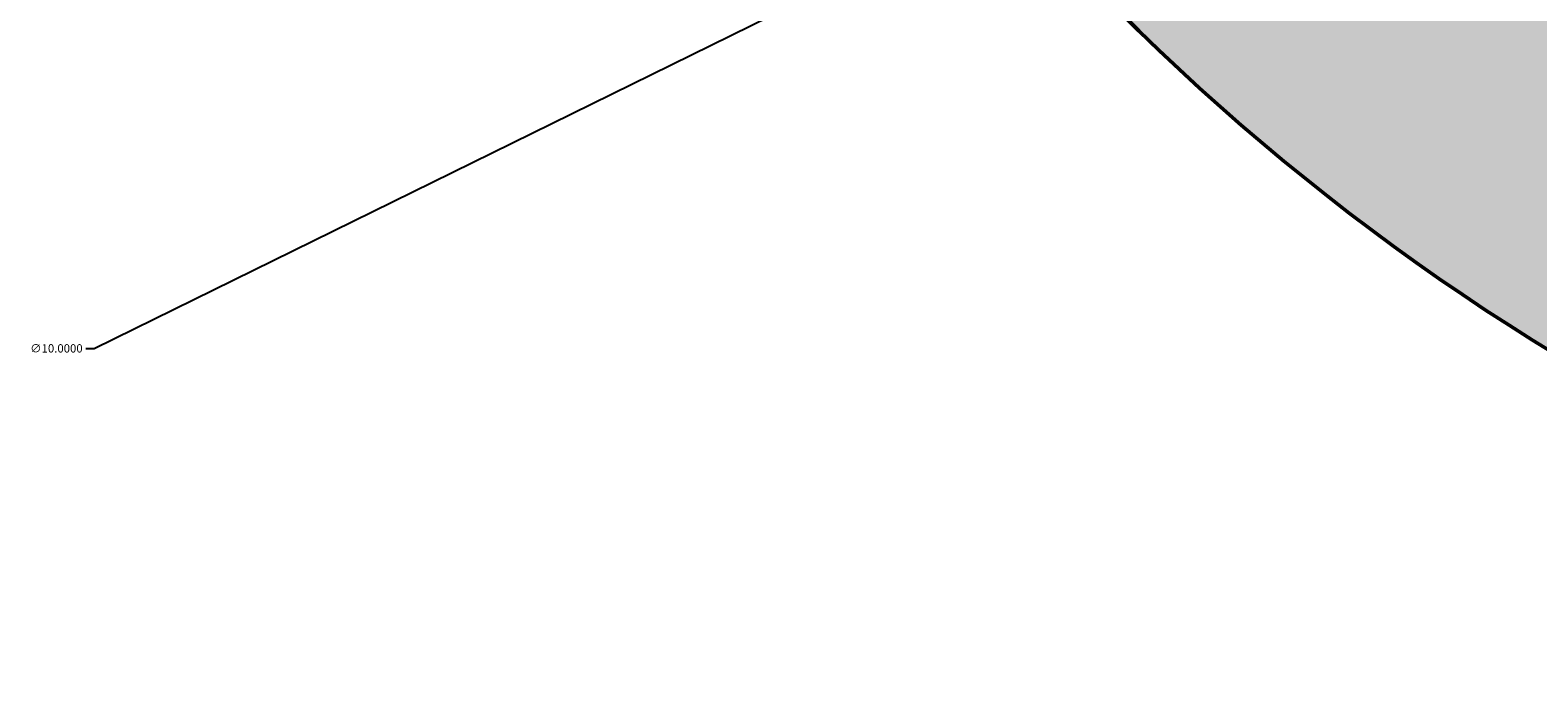
# Model space of a CAD drawing. Units: inches. Extents: x 139261 to 139415, y 52839 to 52963.
# Tile 1 of 20: x 139282 to 139314, y 52850 to 52864. Entities that reach past the tile are written whole.
import ezdxf

# ---------------------------------------------------------------- set-up
doc = ezdxf.new("R2010")
doc.units = ezdxf.units.IN
doc.header["$MEASUREMENT"] = 0
for name, color, linetype, lineweight in [('M-DIMS', 2, 'Continuous', 25), ('M-HATC', 8, 'Continuous', 18), ('M-OUTL', 7, 'Continuous', 50)]:
    doc.layers.add(name, color=color, linetype=linetype, lineweight=lineweight)
doc.styles.get("Standard").update_dxf_attribs({"font": 'arial.ttf'})
doc.dimstyles.get("Standard").update_dxf_attribs({"dimtxt": 0.18, "dimasz": 0.18, "dimexe": 0.18, "dimexo": 0.0625, "dimgap": 0.09, "dimtad": 0, "dimtih": 1, "dimtoh": 1, "dimdec": 4, "dimzin": 0, "dimdsep": 46, "dimtxsty": 'Standard', "dimcen": 0.09, "dimadec": 0, "dimazin": 0, "dimtfac": 1, "dimtdec": 4, "dimtofl": 0, "dimtmove": 0, "dimatfit": 3, "dimfxl": 1, "dimtolj": 1, "dimtzin": 0, "dimarcsym": 0})

# ---------------------------------------------------------------- blocks, each defined once
blk = doc.blocks.new('*D7')
at = {"layer": 'Defpoints', "color": 0, "transparency": 16777216}
for p in [(139316.56, 52874.138), (139307.585, 52869.728)]:
    blk.add_point(p, dxfattribs=at)
at = {"layer": 'M-DIMS', "color": 0, "lineweight": -2, "transparency": 16777216}
for p, q in [((139312.073, 52871.843), (139312.073, 52872.023)), ((139311.983, 52871.933), (139312.163, 52871.933)), ((139282.904, 52857.598), (139307.424, 52869.649)), ((139282.724, 52857.598), (139282.904, 52857.598))]:
    blk.add_line(p, q, dxfattribs=at)
at = {"layer": 'M-DIMS', "color": 0, "transparency": 16777216}
blk.add_solid([(139307.41, 52869.675), (139307.437, 52869.622), (139307.585, 52869.728)], dxfattribs=at)
at = {"layer": 'M-DIMS', "color": 0, "transparency": 16777216, "insert": (139282.093, 52857.598), "char_height": 0.18, "attachment_point": 5}
blk.add_mtext('\\A1;∅10.0000', dxfattribs=at)

msp = doc.modelspace()

# ---------------------------------------------------------------- hatches: boundary and pattern name
at = {"layer": 'M-HATC'}
h = msp.add_hatch(color=256, dxfattribs=at)
h.dxf.hatch_style = 1
h.paths.add_polyline_path([(139290.35689, 52900.21749, 1), (139390.35689, 52900.21749, 1)])
h.paths.add_polyline_path([(139335.36666, 52939.90499, -0.01563646), (139335.35689, 52940.21749, -1), (139345.35689, 52940.21749, -0.01563646), (139345.34711, 52939.90499, -0.13461315), (139364.89157, 52931.80941, -0.691035), (139373.64116, 52928.50176, -0.21521822), (139371.94881, 52924.75216, -0.13461315), (139380.04439, 52905.20771, -0.43265224), (139385.35689, 52900.21749, -0.43265224), (139380.04439, 52895.22726, -0.13461315), (139371.94881, 52875.68281, -0.21521822), (139373.64116, 52871.93321, -0.691035), (139364.89157, 52868.62556, -0.13461315), (139345.34711, 52860.52999, -0.01563646), (139345.35689, 52860.21749, -1), (139335.35689, 52860.21749, -0.01563646), (139335.36666, 52860.52999, -0.13461315), (139315.82221, 52868.62556, -0.691035), (139307.07262, 52871.93321, -0.21521822), (139308.76496, 52875.68281, -0.13461315), (139300.66939, 52895.22726, -0.43265224), (139295.35689, 52900.21749, -0.43265224), (139300.66939, 52905.20771, -0.13461315), (139308.76496, 52924.75216, -0.21521822), (139307.07262, 52928.50176, -0.691035), (139315.82221, 52931.80941, -0.13461315)], flags=16)
h.paths.add_polyline_path([(139365.35689, 52900.21749, -1), (139315.35689, 52900.21749, -1)], flags=0)
h.paths.add_polyline_path([(139323.71474, 52911.30978), (139356.99903, 52911.30978, -0.3027197), (139356.99903, 52889.12519), (139323.71474, 52889.12519, -0.3027197)], flags=0)
h.paths.add_polyline_path([(139364.89157, 52931.80941, 0.13461315), (139345.34711, 52939.90499, -0.93933644), (139335.36666, 52939.90499, 0.13461315), (139315.82221, 52931.80941, -0.18270763), (139317.07262, 52928.50176, -0.64579494), (139308.76496, 52924.75216, 0.13461315), (139300.66939, 52905.20771, -0.39601219), (139305.35689, 52900.21749, -0.39601219), (139300.66939, 52895.22726, 0.13461315), (139308.76496, 52875.68281, -0.64579494), (139317.07262, 52871.93321, -0.18270763), (139315.82221, 52868.62556, 0.13461315), (139335.36666, 52860.52999, -0.93933644), (139345.34711, 52860.52999, 0.13461315), (139364.89157, 52868.62556, -0.18270763), (139363.64116, 52871.93321, -0.64579494), (139371.94881, 52875.68281, 0.13461315), (139380.04439, 52895.22726, -0.39601219), (139375.35689, 52900.21749, -0.39601219), (139380.04439, 52905.20771, 0.13461315), (139371.94881, 52924.75216, -0.64579494), (139363.64116, 52928.50176, -0.18270763)], flags=0)

# ---------------------------------------------------------------- linework, layer by layer
at = {"layer": 'M-OUTL'}
msp.add_circle((139340.35689, 52900.21749), 50, dxfattribs=at)

# ---------------------------------------------------------------- dimensions: what is measured, and where the dimension line sits
at = {"layer": 'M-DIMS'}
dim = msp.add_diameter_dim_2p(p1=(139316.56001, 52874.1385), p2=(139307.58522, 52869.72793), dimstyle='Standard', override={"dimclrd": 0, "dimclre": 0, "dimclrt": 0}, dxfattribs=at)
dim.commit()
dim.dimension.update_dxf_attribs({"geometry": '*D7', "text_midpoint": (139282.09259, 52857.59849), "dimtype": 163})

doc.saveas('drawing.dxf')
